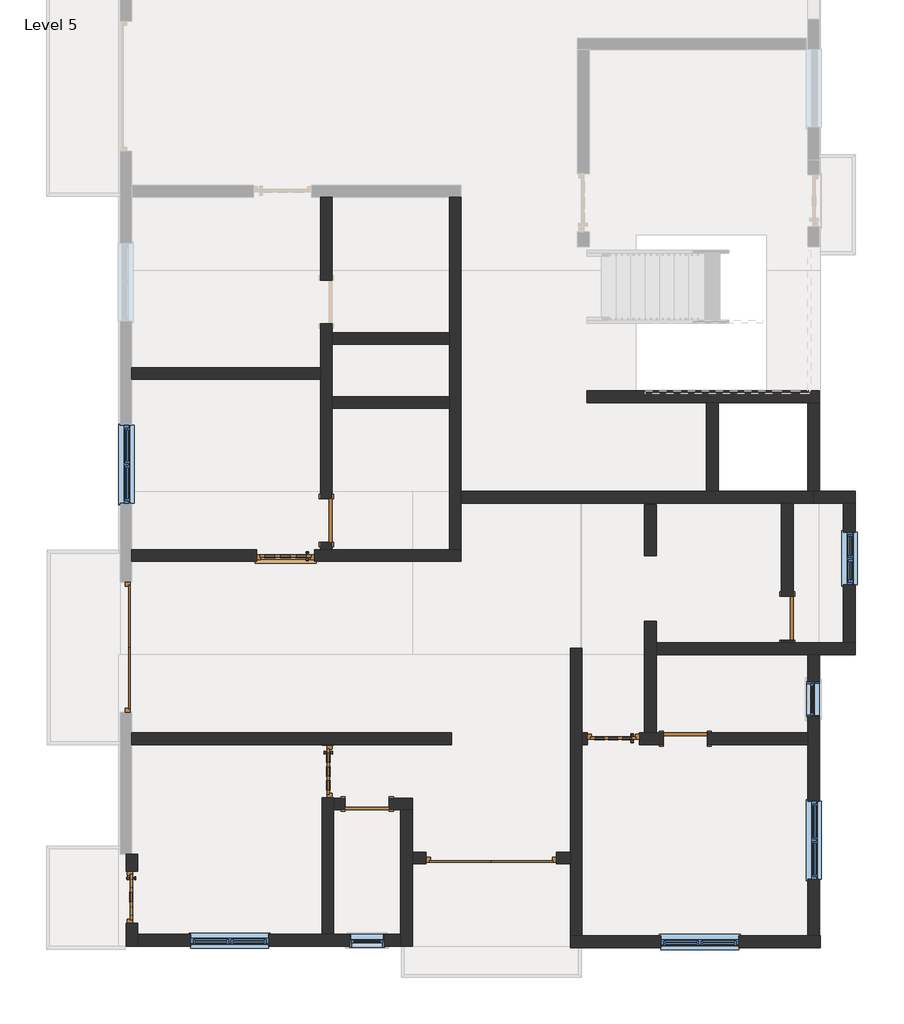
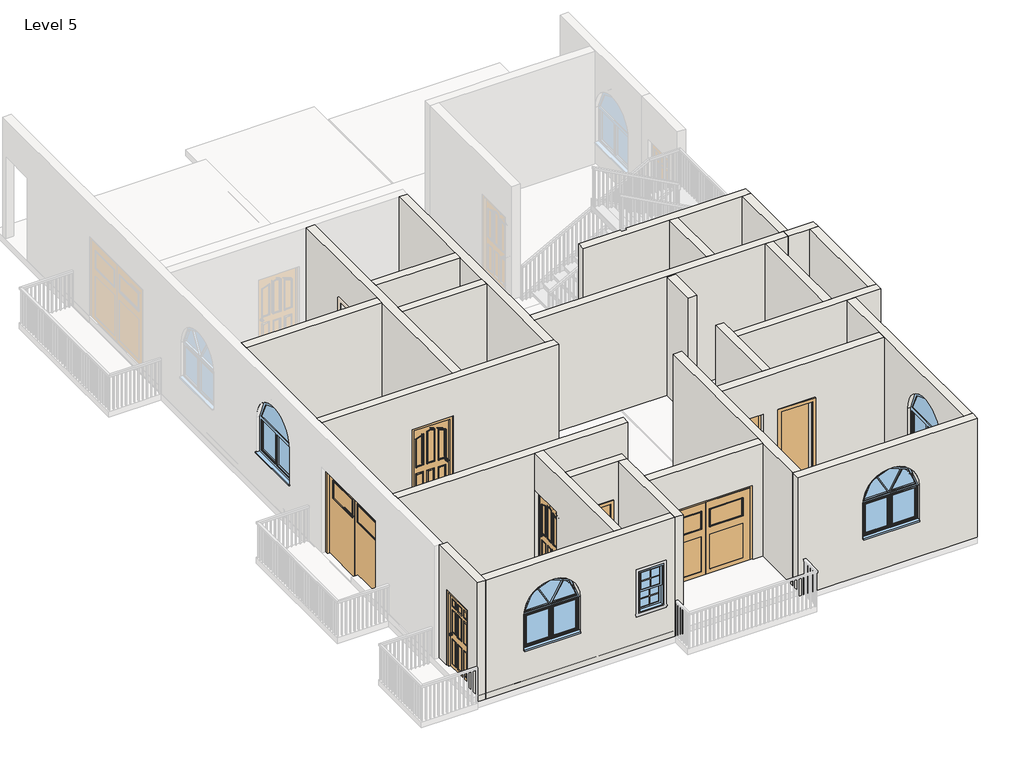
# One storey, part 1 of 7: 27 walls, 10 doors, 7 windows.
# Revit data of these elements (continued)
# Type "Single-Flush : 30\" x 80\"" (continued)
#   Construction Type Id = "MDOOR"
#   Assembly Code = "C1020"
#   Analytic Construction = "Metal"
#   Thickness = 0' - 2"
#   Heat Transfer Coefficient (U) = 0.651978 BTU/(h·ft²·°F)
#   Height = 6' - 8"
#   Trim Projection Ext = 0' - 1"
#   Trim Projection Int = 0' - 1"
#   Trim Width = 0' - 3"
#   Width = 2' - 6"
#   Define Thermal Properties by = 1
#   Define Thermal Properties by = 1
#   Door Material = Door - Panel
#   Frame Material = Door - Frame
#   Visual Light Transmittance = 0
#   Solar Heat Gain Coefficient = 0
#   Function = (empty or 0)
#   Wall Closure = (empty or 0)
# Type "Generic - 9\" w"
#   Assembly Code = "B2010"
#   Layers, outside or top first: 0' - 8" no material (function 1)
# Type "Generic -4.5\" p"
#   Assembly Code = "B2010"
#   Layers, outside or top first: 0' - 8" no material (function 1)
# Type "Window-Double-Hung : 24\" x 42\""
#   Type Mark = "10"
#   Fire Rating = "0.5h"
#   Construction Type Id = "DG-DR"
#   Assembly Code = "B2020100"
#   Analytic Construction = "Double glazing - domestic"
#   Wall Thickness [instance default] = 0' - 6"
#   Window Inset [instance default] = 0' - 0"
#   Visual Light Transmittance = 0.81
#   Thermal Resistance (R) = 1.8146 (h·ft²·°F)/BTU
#   Solar Heat Gain Coefficient = 0.76
#   Muntin Width = 1' - 6"
#   Muntin Height = 1' - 5 1/8"
#   Interior Wall Closure [instance default] = 0' - 1 1/2"
#   Rough Width = 2' - 0 1/2"
#   Rough Height = 3' - 6 1/2"
#   Frame Extension [instance default] = 0' - 1 1/4"
#   Exterior Wall Closure [instance default] = 0' - 0 1/2"
#   Extension Jamb [instance default] = 0' - 1 1/2"
#   Heat Transfer Coefficient (U) = 0.5511 BTU/(h·ft²·°F)
#   Height = 3' - 6"
#   Width = 2' - 0"
#   Define Thermal Properties by = 1
#   Top Muntin Visibility = yes
#   Indicator Visibility [instance default] = yes
#   Extension Jamb Visibility [instance default] = yes
#   Interior Trim Visibility [instance default] = yes
#   Exterior Trim Visibility [instance default] = yes
#   Define Thermal Properties by = 1
#   Bottom Muntin Visibility = yes
#   Muntin Pattern = Muntin Pattern_2x2 : Muntin Pattern_2x2
#   Interior Trim Material = Wood - Stained
#   Interior Trim = Trim-Window-Interior-Flat : Picture Frame
#   Exterior Trim Material = Clad - White
#   Exterior Trim = Trim-Window-Exterior-Flat : with Sill
#   Glass Panel Material = Glass
#   Exterior Frame Material = Clad - White
#   Interior Frame Material = Wood - Stained
#   Wall Closure = (empty or 0)
# Type "Windows_Arched : 1360x910mm"
#   Type Mark = "20"
#   Operation = "UserDefined"
#   Construction Type Id = "GSP4R"
#   Manufacturer = "Revit"
#   Keynote = "L10"
#   Analytic Construction = "1/8 in Pilkington single glazing"
#   Wrap Layers (Ext) from Ext = 0' - 4.03543"
#   Wrap Layers (Int) from Ext = 0' - 6.98819"
#   Window Board Projection = 0' - 0.98425"
#   Window Board Extension = 0' - 0.98425"
#   Visual Light Transmittance = 0.9
#   Solar Heat Gain Coefficient = 0.78
#   Rough Width = 4' - 5.54331"
#   Rough Height = 2' - 11.82677"
#   Height = 2' - 11.82677"
#   Width = 4' - 5.54331"
#   Heat Transfer Coefficient (U) = 0.6496 BTU/(h·ft²·°F)
#   Glazing Thickness = 0' - 0.94488"
#   FrameOffset - External = 0' - 1.9685"
#   Frame Depth = 0' - 2.67717"
#   Default Head Height = 6' - 11.07087"
#   Cill Depth = 0' - 3.44488"
#   Cavity Closer Width = 0' - 1.9685"
#   Cavity Closer Offset from Ext = 0' - 4.03543"
#   Cavity Closer Depth = 0' - 3.34646"
#   Vis - Cavity Closers = yes
#   Define Thermal Properties by = 1
#   Material Trim = Window Frame
#   Material Glass = Glass
#   Material Frame = Window Frame
#   Wall Closure = (empty or 0)
# Type "Windows_Dbl_w-Glazing_Bars : 910x910mm"
#   Type Mark = "33"
#   Operation = "DoublePanelVertical"
#   Construction Type Id = "GSP4R"
#   Manufacturer = "Revit"
#   Keynote = "L10"
#   Analytic Construction = "1/8 in Pilkington single glazing"
#   Wrap Layers (Ext) from Ext = 0' - 4.03543"
#   Wrap Layers (Int) from Ext = 0' - 6.98819"
#   Window Board Projection = 0' - 0.98425"
#   Window Board Extension = 0' - 0.98425"
#   Visual Light Transmittance = 0.9
#   Solar Heat Gain Coefficient = 0.78
#   Rough Width = 2' - 11.82677"
#   Rough Height = 2' - 11.82677"
#   Height = 2' - 11.82677"
#   Width = 2' - 11.82677"
#   Heat Transfer Coefficient (U) = 0.6496 BTU/(h·ft²·°F)
#   Glazing Thickness = 0' - 0.94488"
#   Glazing Bar Thickness = 0' - 0.7874"
#   FrameOffset - External = 0' - 1.9685"
#   Frame Depth = 0' - 2.55906"
#   Default Head Height = 6' - 10.67717"
#   Cill Depth = 0' - 3.44488"
#   Cavity Closer Width = 0' - 1.9685"
#   Cavity Closer Offset from Ext = 0' - 4.03543"
#   Cavity Closer Depth = 0' - 3.34646"
#   Vis - Glazing Bars = yes
#   Vis - Cavity Closers = yes
#   Define Thermal Properties by = 1
#   Material Trim = Window Frame
#   Material Glazing Bars = Window Frame
#   Material Glass = Glass
#   Material Frame = Window Frame
#   Wall Closure = (empty or 0)
# Element 1 (IfcDoor, "Doors_ExtSgl_5 : 910x2110mm")
#   Phase Created = New Construction
#   Materials on its faces: "Door - Panel", "Door - Handle", "Door - Frame/Mullion", "Door - Glazing"
# Element 2 (IfcDoor, "Doors_ExtSgl_6 : 1010x2110mm")
#   Phase Created = New Construction
#   Materials on its faces: "Door - Panel", "Door - Handle", "Door - Frame/Mullion", "Door - Glazing"
# Elements 3, 4 (IfcDoor, "Doors_ExtSgl_6 : 910x2110mm")
#   Phase Created = New Construction
#   Materials on its faces: "Door - Panel", "Door - Handle", "Door - Frame/Mullion", "Door - Glazing"
# Element 5 (IfcDoor, "Doors_Garage_Timber_Side_Hung_Glazing : 2270x2050mm")
#   Phase Created = New Construction
#   Materials on its faces: "Door - Panel", "Door - Frame/Mullion", "Door - Glazing"
# Element 6 (IfcDoor, "Doors_Garage_Timber_Side_Hung_Glazing : 2270x2200mm")
#   Phase Created = New Construction
#   Materials on its faces: "Door - Panel", "Door - Frame/Mullion", "Door - Glazing"
# Elements 7, 8, 9, 10 (IfcDoor, "Single-Flush : 30\" x 80\"")
#   Phase Created = New Construction
#   Materials on its faces: "Door - Frame", "Door - Panel"
# Element 11 (IfcWall, "Generic - 9\" w")
#   Top Offset = 0' - 0"
#   Base Offset = 0' - 0"
#   wall height = 10' - 0"
#   Phase Created = New Construction
#   Base Constraint = Level 5
#   Top Constraint = Level 6
#   Materials on its faces: "Default Wall", "Door - Frame", "Earth"
# Elements 12, 13 (IfcWall, "Generic - 9\" w")
#   Top Offset = 0' - 0"
#   Base Offset = 0' - 0"
#   wall height = 10' - 0"
#   Phase Created = New Construction
#   Base Constraint = Level 5
#   Top Constraint = Level 6
#   Materials on its faces: "Default Wall"
# Element 14 (IfcWall, "Generic - 9\" w")
#   Top Offset = 0' - 0"
#   Base Offset = 0' - 0"
#   wall height = 10' - 0"
#   Phase Created = New Construction
#   Base Constraint = Level 5
#   Top Constraint = Level 6
#   Materials on its faces: "Default Wall", "Door - Frame/Mullion", "Earth"
# Element 15 (IfcWall, "Generic - 9\" w")
#   Top Offset = 0' - 0"
#   Base Offset = 0' - 0"
#   wall height = 10' - 0"
#   Phase Created = New Construction
#   Base Constraint = Level 5
#   Top Constraint = Level 6
#   Materials on its faces: "Default Wall", "Concrete, Lightweight", "Wood - Stained"
# Element 16 (IfcWall, "Generic - 9\" w")
#   Top Offset = 0' - 0"
#   Base Offset = 0' - 0"
#   wall height = 10' - 0"
#   Phase Created = New Construction
#   Base Constraint = Level 5
#   Top Constraint = Level 6
#   Materials on its faces: "Default Wall", "Wood - Stained"
# Element 17 (IfcWall, "Generic - 9\" w")
#   Top Offset = 0' - 0"
#   Base Offset = 0' - 0"
#   wall height = 10' - 0"
#   Phase Created = New Construction
#   Base Constraint = Level 5
#   Top Constraint = Level 6
#   Materials on its faces: "Default Wall", "Earth"
# Elements 18, 19 (IfcWall, "Generic - 9\" w")
#   Top Offset = 0' - 0"
#   Base Offset = 0' - 0"
#   wall height = 10' - 0"
#   Phase Created = New Construction
#   Base Constraint = Level 5
#   Top Constraint = Level 6
#   Materials on its faces: "Default Wall", "Concrete, Lightweight"
# Elements 20, 21, 22, 23, 24, 25, 26, 27, 28, 31, 32, 33, 36, 37 (IfcWall, "Generic -4.5\" p")
#   Top Offset = 0' - 0"
#   Base Offset = 0' - 0"
#   wall height = 10' - 0"
#   Phase Created = New Construction
#   Base Constraint = Level 5
#   Top Constraint = Level 6
#   Materials on its faces: "Default Wall"
# Element 29 (IfcWall, "Generic -4.5\" p")
#   Top Offset = 0' - 0"
#   Base Offset = 0' - 0"
#   wall height = 10' - 0"
#   Phase Created = New Construction
#   Base Constraint = Level 5
#   Top Constraint = Level 6
#   Materials on its faces: "Default Wall", "Concrete, Lightweight"
# Element 30 (IfcWall, "Generic -4.5\" p")
#   Top Offset = 0' - 0"
#   Base Offset = 0' - 0"
#   wall height = 10' - 0"
#   Phase Created = New Construction
#   Base Constraint = Level 5
#   Top Constraint = Level 6
#   Materials on its faces: "Default Wall", "Door - Frame/Mullion"
# Elements 34, 35 (IfcWall, "Generic -4.5\" p")
#   Top Offset = 0' - 0"
#   Base Offset = 0' - 0"
#   wall height = 10' - 0"
#   Phase Created = New Construction
#   Base Constraint = Level 5
#   Top Constraint = Level 6
#   Materials on its faces: "Default Wall", "Earth"
# Element 38 (IfcWindow, "Window-Double-Hung : 24\" x 42\"")
#   Mark = "61"
#   Window Inset = 0' - 0"
#   Interior Wall Closure = 0' - 1 1/2"
#   Frame Extension = 0' - 1 1/4"
#   Exterior Wall Closure = 0' - 0 1/2"
#   Interior Trim Visibility = yes
#   Indicator Visibility = yes
#   Exterior Trim Visibility = yes
#   Phase Created = New Construction
#   Materials on its faces: "Wood - Stained", "Glass", "Clad - White"
# Element 39 (IfcWindow, "Window-Double-Hung : 24\" x 42\"")
#   Mark = "91"
#   Window Inset = 0' - 0"
#   Interior Wall Closure = 0' - 1 1/2"
#   Frame Extension = 0' - 1 1/4"
#   Exterior Wall Closure = 0' - 0 1/2"
#   Interior Trim Visibility = yes
#   Indicator Visibility = yes
#   Exterior Trim Visibility = yes
#   Phase Created = New Construction
#   Materials on its faces: "Wood - Stained", "Glass", "Clad - White"
# Element 40 (IfcWindow, "Windows_Arched : 1360x910mm")
#   Mark = "57"
#   Phase Created = New Construction
#   Materials on its faces: "Window Frame", "Glass"
# Element 41 (IfcWindow, "Windows_Arched : 1360x910mm")
#   Mark = "58"
#   Phase Created = New Construction
#   Materials on its faces: "Window Frame", "Glass"
# Element 42 (IfcWindow, "Windows_Arched : 1360x910mm")
#   Mark = "59"
#   Phase Created = New Construction
#   Materials on its faces: "Window Frame", "Glass"
# Element 43 (IfcWindow, "Windows_Arched : 1360x910mm")
#   Mark = "86"
#   Phase Created = New Construction
#   Materials on its faces: "Window Frame", "Glass"
# Element 44 (IfcWindow, "Windows_Dbl_w-Glazing_Bars : 910x910mm")
#   Mark = "62"
#   Phase Created = New Construction
#   Materials on its faces: "Window Frame", "Glass"
# Materials
#   "Door - Glazing": colour RGB 0 0 255, transparency 0.75
#   "Door - Panel": class "Wood", colour RGB 210 159 95, transparency 0, Cost = 0
#   "Door - Frame/Mullion": class "Wood", colour RGB 212 179 113, transparency 0
#   "Door - Handle": colour RGB 0 0 0, transparency 0
#   "Door - Frame": colour RGB 118 70 51, transparency 0, Cost = 0
#   "Wood - Stained": class "Wood", colour RGB 224 178 126, transparency 0, Cost = 0
#   "Clad - White": class "Wood", colour RGB 242 242 238, transparency 0, Cost = 0
#   "Glass": class "Glass", colour RGB 0 128 192, transparency 0.75, Description = "Soda Lime Glass", Cost = 0
#   "Window Frame": colour RGB 249 249 249, transparency 0
#   "Default Wall": colour RGB 128 128 128, transparency 0, Cost = 0
#   "Earth": class "Generic", colour RGB 97 75 62, transparency 0, Description = "Soil", Cost = 0
#   "Concrete, Lightweight": class "Concrete", colour RGB 142 141 140, transparency 0, Description = "Lightweight concrete", Cost = 0
